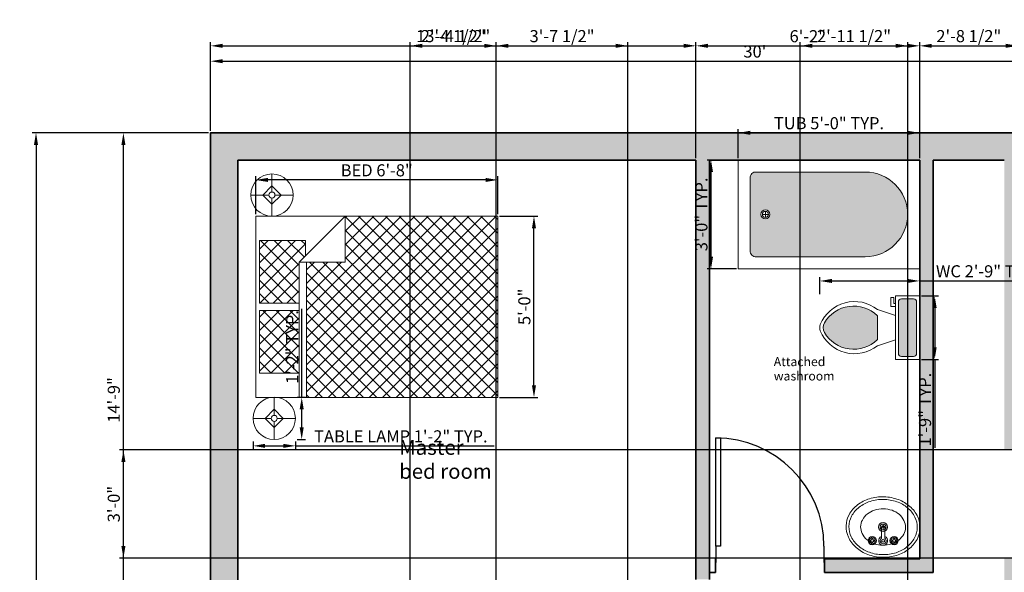
# Model space of a CAD drawing. Units: inches. Extents: x 1872 to 2380, y 714 to 1327.
# Tile 8 of 9: x 1872 to 2198, y 1144 to 1327. Entities that reach past the tile are written whole.
import ezdxf

# ---------------------------------------------------------------- set-up
doc = ezdxf.new("R2010")
doc.units = ezdxf.units.IN
for name, color, linetype, lineweight in [('A-ANNO-DIMS', 2, 'Continuous', 18), ('A-AREA-IDEN', 7, 'Continuous', 18), ('A-DOOR', 4, 'Continuous', 25), ('A-FLOR-FIXT', 9, 'Continuous', 20), ('A-FURN', 8, 'Continuous', 18), ('A-WALL', 7, 'Continuous', 35)]:
    doc.layers.add(name, color=color, linetype=linetype, lineweight=lineweight)
for name, color, linetype, lineweight, true_color in [('A-FLOR-FIXT-PATT', 7, 'Continuous', 13, 0xd1ffff), ('A-FURN-PATT', 254, 'Continuous', 13, 0xf8ceb3), ('A-WALL-PATT', 242, 'Continuous', 13, 0xd52e31)]:
    doc.layers.add(name, color=color, linetype=linetype, lineweight=lineweight, true_color=true_color)
doc.styles.get("Standard").update_dxf_attribs({"font": 'arial.ttf'})
doc.dimstyles.new('ISO-25', dxfattribs={"dimtxt": 4, "dimasz": 4, "dimexe": 1.25, "dimexo": 0.625, "dimtad": 1, "dimdec": 0, "dimlunit": 3, "dimtxsty": 'Standard', "dimcen": 2.5, "dimadec": 0, "dimazin": 0, "dimtfac": 1, "dimtdec": 0, "dimtmove": 0, "dimatfit": 3, "dimfxl": 1, "dimarcsym": 0})

# ---------------------------------------------------------------- blocks, each defined once
blk = doc.blocks.new('*U3')
for p, q in [((0, 0), (0, -6)), ((40, 0), (40, -6))]:
    blk.add_line(p, q)
blk.add_lwpolyline([(0, 0), (0, 40), (1.75, 40), (1.75, 0)], close=True)
blk.add_arc((0, 0), 40, 0, 90)
blk = doc.blocks.new('Bed - Queen')
for p, q in [((0, -80.00003), (0, 0)), ((0, 0), (59.99999, 0)), ((59.99999, 0), (59.99999, -80.00003)), ((7.99999, -1.2), (28.79998, -1.2)), ((7.99999, -14.4), (7.99999, -1.2)), ((28.79998, -1.2), (28.79998, -14.4)), ((31.19999, -1.2), (51.99999, -1.2)), ((31.19999, -14.4), (31.19999, -1.2)), ((51.99999, -1.2), (51.99999, -16.4)), ((0, -14.4), (44.8, -14.4)), ((59.99999, -29.6), (44.8, -14.4)), ((44.8, -14.4), (44.8, -29.6)), ((44.8, -16.8), (0, -16.8)), ((51.99999, -16.4), (46.79936, -16.4)), ((44.8, -29.6), (59.99999, -29.6)), ((59.99999, -80.00003), (0, -80.00003))]:
    blk.add_line(p, q)
blk = doc.blocks.new('Lamp - Table')
for p, q in [((0, 7), (0, 1)), ((-1, 0), (-7, 0)), ((0, 3), (-3, 0)), ((-3, 0), (0, -3)), ((3, 0), (0, 3)), ((0, -3), (3, 0)), ((1, 0), (7, 0)), ((0, -1), (0, -7))]:
    blk.add_line(p, q)
for radius in [7, 1]:
    blk.add_circle((0, 0), radius)
blk = doc.blocks.new('Bath Tub - 26 x 60 in.')
for p, q in [((8, -18), (10, -18)), ((9, -17), (9, -19))]:
    blk.add_line(p, q)
blk.add_lwpolyline([(0, -36), (0, 0), (60, 0), (60, -36)], close=True)
for points in [[(4, -30), (4, -6)], [(6, -4), (42, -4)], [(42, -32), (6, -32)]]:
    blk.add_lwpolyline(points)
for radius in [1.5, 1]:
    blk.add_circle((9, -18), radius)
for centre, radius, start, end in [((5.75, -5.75), 1.77, 81.8699, 188.1301), ((42, -18), 14, 270, 90), ((5.75, -30.25), 1.77, 171.8699, 278.1301)]:
    blk.add_arc(centre, radius, start, end)
blk = doc.blocks.new('Toilet - top')
for p, q in [((9.5, -6), (9.5, -2)), ((-10, -8.5), (-8, -8.5)), ((-10, -9.5), (-10, -8.5)), ((-7, -9.5), (-10, -9.5)), ((-8, -8.5), (-8, -8)), ((-7, -8), (-7, -9.5)), ((-4, -8), (-6, -14)), ((4, -8), (6, -14)), ((4, -14), (-4, -14))]:
    blk.add_line(p, q)
blk.add_lwpolyline([(10.5, -8), (10.5, 0), (-10.5, 0), (-10.5, -8)], close=True)
for points in [[(-9.5, -2), (-9.5, -6)], [(8.5, -1), (-8.5, -1)], [(-8.5, -7), (8.5, -7)]]:
    blk.add_lwpolyline(points)
for centre, radius, start, end in [((-8.62, -1.88), 0.884, 81.8699, 188.1301), ((8.62, -1.88), 0.884, 351.8699, 98.1301), ((-8.62, -6.12), 0.884, 171.8699, 278.1301), ((8.62, -6.12), 0.884, 261.8699, 8.1301), ((3.52, -21.58), 12.17, 141.4691, 247.9714), ((4.2, -21.82), 11.33, 136.3677, 238.9468), ((-3.52, -21.58), 12.17, 292.0284, 38.5307), ((-4.2, -21.82), 11.33, 301.053, 43.6321), ((0, -27.88), 4, 245.7318, 294.2682), ((0, -29), 4, 254.8605, 285.1395)]:
    blk.add_arc(centre, radius, start, end)
blk = doc.blocks.new('Sink - Oval top')
for p, q in [((-1, 0), (1, 0)), ((0, 1), (0, -1))]:
    blk.add_line(p, q)
for points in [[(-12.23, 0.39, 0.117634), (-11.46, -3.36, 0.104469), (-8.88, -6.8, 0.090016), (-5.08, -9.07, 0.08192), (-0.32, -10.02, 0.08192), (4.49, -9.38, 0.090016), (8.42, -7.36, 0.104469), (11.22, -4.09, 0.117634), (12.23, -0.39, 0.117634), (11.46, 3.36, 0.104469), (8.88, 6.8, 0.090016), (5.08, 9.07, 0.08192), (0.32, 10.02, 0.08192), (-4.49, 9.38, 0.090016), (-8.42, 7.36, 0.104469), (-11.22, 4.09, 0.117634)], [(-11.29, 0.16, 0.118622), (-10.52, -3.25, 0.104678), (-8.07, -6.36, 0.089562), (-4.54, -8.37, 0.081185), (-0.13, -9.15, 0.081185), (4.3, -8.49, 0.089562), (7.89, -6.58, 0.104678), (10.42, -3.55, 0.118622), (11.29, -0.16, 0.118622), (10.52, 3.25, 0.104678), (8.07, 6.36, 0.089562), (4.54, 8.37, 0.081185), (0.13, 9.15, 0.081185), (-4.3, 8.49, 0.089562), (-7.89, 6.58, 0.104678), (-10.42, 3.55, 0.118622)], [(-7.42, 0.08, 0.118283), (-6.91, -2.17, 0.104607), (-5.29, -4.21, 0.089718), (-2.97, -5.53, 0.081436), (-0.07, -6.04, 0.081436), (2.84, -5.59, 0.089718), (5.2, -4.33, 0.104607), (6.86, -2.32, 0.118283), (7.42, -0.08, 0.118283), (6.91, 2.17, 0.104607), (5.29, 4.21, 0.089718), (2.97, 5.53, 0.081436), (0.07, 6.04, 0.081436), (-2.84, 5.59, 0.089718), (-5.2, 4.33, 0.104607), (-6.86, 2.32, 0.118283)]]:
    blk.add_lwpolyline(points, format="xyb", close=True)
for radius in [1.5, 1]:
    blk.add_circle((0, 0), radius)
blk = doc.blocks.new('Faucet - Bathroom top')
for p, q in [((-4.107, 0.125), (-4.375, 0.125)), ((-3.75, 0.4788), (-3.75, 0.75)), ((-3.5, 0.482), (-3.5, 0.75)), ((-3.1461, 0.125), (-2.875, 0.125)), ((3.143, 0.125), (2.875, 0.125)), ((3.5, 0.4788), (3.5, 0.75)), ((3.75, 0.482), (3.75, 0.75)), ((4.1039, 0.125), (4.375, 0.125)), ((-4.1039, -0.125), (-4.375, -0.125)), ((-3.75, -0.4821), (-3.75, -0.75)), ((-3.5, -0.4789), (-3.5, -0.75)), ((-3.143, -0.125), (-2.875, -0.125)), ((-0.5, -0.8639), (-0.5, -4.5)), ((0.5, -4.5), (0.5, -0.8631)), ((3.1461, -0.125), (2.875, -0.125)), ((3.5, -0.4821), (3.5, -0.75)), ((3.75, -0.4789), (3.75, -0.75)), ((4.107, -0.125), (4.375, -0.125))]:
    blk.add_line(p, q)
for centre, radius in [((-3.625, 0), 1.375), ((-4.625, 0), 0.2795), ((-3.625, 0), 0.5), ((-3.625, 1), 0.2795), ((-2.625, 0), 0.2795), ((0, 0), 0.5), ((3.625, 0), 1.375), ((2.625, 0), 0.2795), ((3.625, 0), 0.5), ((3.625, 1), 0.2795), ((4.625, 0), 0.2795), ((-3.625, -1), 0.2795), ((3.625, -1), 0.2795)]:
    blk.add_circle(centre, radius)
for centre, radius, start, end in [((-3.625, 0), 1, 105.2407, 164.2093), ((-3.625, 0), 1, 16.44125, 74.07887), ((0, 0), 1.5, 289.6514, 250.3603), ((0, 0), 1, 300.3431, 239.7554), ((3.625, 0), 1, 106.12, 164.0884), ((3.625, 0), 1, 16.23422, 73.90469), ((-3.625, 0), 1, 196.2342, 253.9047), ((-3.625, 0), 1, 286.12, 344.0884), ((3.625, 0), 1, 196.4413, 254.0789), ((3.625, 0), 1, 285.2407, 344.2093), ((0, -4.5), 0.5, 180, 0)]:
    blk.add_arc(centre, radius, start, end)
blk = doc.blocks.new('*D22')
at = {"layer": 'A-ANNO-DIMS', "color": 0, "lineweight": -2, "transparency": 16777216}
for p, q in [((1935.4, 1290.27), (1935.4, 1314.61)), ((1939.4, 1313.36), (2291.4, 1313.36)), ((2295.4, 1290.27), (2295.4, 1314.61))]:
    blk.add_line(p, q, dxfattribs=at)
at = {"layer": 'A-ANNO-DIMS', "color": 0, "transparency": 16777216}
for points in [[(1939.4, 1314.03), (1939.4, 1312.69), (1935.4, 1313.36)], [(2291.4, 1314.03), (2291.4, 1312.69), (2295.4, 1313.36)]]:
    blk.add_solid(points, dxfattribs=at)
at = {"layer": 'Defpoints', "color": 0, "transparency": 16777216}
for p in [(2295.4, 1313.36), (1935.4, 1289.64), (2295.4, 1289.64)]:
    blk.add_point(p, dxfattribs=at)
at = {"layer": 'A-ANNO-DIMS', "color": 0, "transparency": 16777216, "insert": (2115.4, 1316.03), "char_height": 4, "attachment_point": 5}
blk.add_mtext("30'", dxfattribs=at)
blk = doc.blocks.new('*D23')
at = {"layer": 'A-ANNO-DIMS', "color": 0, "lineweight": -2, "transparency": 16777216}
for p, q in [((1934.77, 1289.64), (1876.44, 1289.64)), ((1877.69, 1285.64), (1877.69, 813.64)), ((1934.77, 809.64), (1876.44, 809.64))]:
    blk.add_line(p, q, dxfattribs=at)
at = {"layer": 'A-ANNO-DIMS', "color": 0, "transparency": 16777216}
for points in [[(1877.02, 1285.64), (1878.36, 1285.64), (1877.69, 1289.64)], [(1877.02, 813.64), (1878.36, 813.64), (1877.69, 809.64)]]:
    blk.add_solid(points, dxfattribs=at)
at = {"layer": 'Defpoints', "color": 0, "transparency": 16777216}
for p in [(1935.4, 1289.64), (1877.69, 809.64), (1935.4, 809.64)]:
    blk.add_point(p, dxfattribs=at)
at = {"layer": 'A-ANNO-DIMS', "color": 0, "transparency": 16777216, "insert": (1875.02, 1049.64), "char_height": 4, "attachment_point": 5, "rotation": 90}
blk.add_mtext("40'", dxfattribs=at)
blk = doc.blocks.new('*D24')
at = {"layer": 'A-ANNO-DIMS', "color": 0, "lineweight": -2, "transparency": 16777216}
for p, q in [((1949.46, 1187.48), (1949.46, 1184.76)), ((1953.46, 1186.01), (1959.46, 1186.01)), ((1963.46, 1187.48), (1963.46, 1184.76)), ((1963.46, 1186.01), (2029.21, 1186.01))]:
    blk.add_line(p, q, dxfattribs=at)
at = {"layer": 'A-ANNO-DIMS', "color": 0, "transparency": 16777216}
for points in [[(1953.46, 1186.68), (1953.46, 1185.34), (1949.46, 1186.01)], [(1959.46, 1186.68), (1959.46, 1185.34), (1963.46, 1186.01)]]:
    blk.add_solid(points, dxfattribs=at)
at = {"layer": 'Defpoints', "color": 0, "transparency": 16777216}
for p in [(1949.46, 1188.11), (1963.46, 1188.11), (1963.46, 1186.01)]:
    blk.add_point(p, dxfattribs=at)
at = {"layer": 'A-ANNO-DIMS', "color": 0, "transparency": 16777216, "insert": (1998.34, 1188.64), "char_height": 4, "attachment_point": 5}
blk.add_mtext('TABLE LAMP 1\'-2" TYP.', dxfattribs=at)
blk = doc.blocks.new('*D25')
at = {"layer": 'A-ANNO-DIMS', "color": 0, "lineweight": -2, "transparency": 16777216}
for p, q in [((1965.56, 1202.11), (1965.56, 1231.37)), ((1964.08, 1202.11), (1966.81, 1202.11)), ((1965.56, 1192.11), (1965.56, 1198.11)), ((1964.08, 1188.11), (1966.81, 1188.11))]:
    blk.add_line(p, q, dxfattribs=at)
at = {"layer": 'A-ANNO-DIMS', "color": 0, "transparency": 16777216}
for points in [[(1964.89, 1198.11), (1966.22, 1198.11), (1965.56, 1202.11)], [(1964.89, 1192.11), (1966.22, 1192.11), (1965.56, 1188.11)]]:
    blk.add_solid(points, dxfattribs=at)
at = {"layer": 'Defpoints', "color": 0, "transparency": 16777216}
for p in [(1963.46, 1202.11), (1965.56, 1202.11), (1963.46, 1188.11)]:
    blk.add_point(p, dxfattribs=at)
at = {"layer": 'A-ANNO-DIMS', "color": 0, "transparency": 16777216, "insert": (1962.92, 1218.74), "char_height": 4, "attachment_point": 5, "rotation": 90}
blk.add_mtext('1\'-2" TYP.', dxfattribs=at)
blk = doc.blocks.new('*D26')
at = {"layer": 'A-ANNO-DIMS', "color": 0, "lineweight": -2, "transparency": 16777216}
for p, q in [((1950.37, 1262.67), (1950.37, 1275.29)), ((2026.37, 1274.04), (1954.37, 1274.04)), ((2030.37, 1262.67), (2030.37, 1275.29))]:
    blk.add_line(p, q, dxfattribs=at)
at = {"layer": 'A-ANNO-DIMS', "color": 0, "transparency": 16777216}
for points in [[(1954.37, 1274.71), (1954.37, 1273.38), (1950.37, 1274.04)], [(2026.37, 1274.71), (2026.37, 1273.38), (2030.37, 1274.04)]]:
    blk.add_solid(points, dxfattribs=at)
at = {"layer": 'Defpoints', "color": 0, "transparency": 16777216}
for p in [(1950.37, 1274.04), (1950.37, 1262.04), (2030.37, 1262.04)]:
    blk.add_point(p, dxfattribs=at)
at = {"layer": 'A-ANNO-DIMS', "color": 0, "transparency": 16777216, "insert": (1990.37, 1276.71), "char_height": 4, "attachment_point": 5}
blk.add_mtext('BED 6\'-8"', dxfattribs=at)
blk = doc.blocks.new('*D27')
at = {"layer": 'A-ANNO-DIMS', "color": 0, "lineweight": -2, "transparency": 16777216}
for p, q in [((2030.99, 1262.04), (2043.62, 1262.04)), ((2042.37, 1206.04), (2042.37, 1258.04)), ((2030.99, 1202.04), (2043.62, 1202.04))]:
    blk.add_line(p, q, dxfattribs=at)
at = {"layer": 'A-ANNO-DIMS', "color": 0, "transparency": 16777216}
for points in [[(2041.7, 1258.04), (2043.03, 1258.04), (2042.37, 1262.04)], [(2041.7, 1206.04), (2043.03, 1206.04), (2042.37, 1202.04)]]:
    blk.add_solid(points, dxfattribs=at)
at = {"layer": 'Defpoints', "color": 0, "transparency": 16777216}
for p in [(2030.37, 1262.04), (2042.37, 1262.04), (2030.37, 1202.04)]:
    blk.add_point(p, dxfattribs=at)
at = {"layer": 'A-ANNO-DIMS', "color": 0, "transparency": 16777216, "insert": (2039.7, 1232.04), "char_height": 4, "attachment_point": 5, "rotation": 90}
blk.add_mtext('5\'-0"', dxfattribs=at)
blk = doc.blocks.new('*D34')
at = {"layer": 'A-ANNO-DIMS', "color": 0, "lineweight": -2, "transparency": 16777216}
for p, q in [((2109.91, 1281.27), (2109.91, 1290.89)), ((2113.91, 1289.64), (2165.91, 1289.64)), ((2169.91, 1281.27), (2169.91, 1290.89))]:
    blk.add_line(p, q, dxfattribs=at)
at = {"layer": 'A-ANNO-DIMS', "color": 0, "transparency": 16777216}
for points in [[(2113.91, 1290.31), (2113.91, 1288.98), (2109.91, 1289.64)], [(2165.91, 1290.31), (2165.91, 1288.98), (2169.91, 1289.64)]]:
    blk.add_solid(points, dxfattribs=at)
at = {"layer": 'Defpoints', "color": 0, "transparency": 16777216}
for p in [(2169.91, 1289.64), (2109.91, 1280.64), (2169.91, 1280.64)]:
    blk.add_point(p, dxfattribs=at)
at = {"layer": 'A-ANNO-DIMS', "color": 0, "transparency": 16777216, "insert": (2139.91, 1292.31), "char_height": 4, "attachment_point": 5}
blk.add_mtext('TUB 5\'-0" TYP.', dxfattribs=at)
blk = doc.blocks.new('*D35')
at = {"layer": 'A-ANNO-DIMS', "color": 0, "lineweight": -2, "transparency": 16777216}
for p, q in [((2109.29, 1280.64), (2099.66, 1280.64)), ((2100.91, 1248.64), (2100.91, 1276.64)), ((2109.29, 1244.64), (2099.66, 1244.64))]:
    blk.add_line(p, q, dxfattribs=at)
at = {"layer": 'A-ANNO-DIMS', "color": 0, "transparency": 16777216}
for points in [[(2100.25, 1276.64), (2101.58, 1276.64), (2100.91, 1280.64)], [(2100.25, 1248.64), (2101.58, 1248.64), (2100.91, 1244.64)]]:
    blk.add_solid(points, dxfattribs=at)
at = {"layer": 'Defpoints', "color": 0, "transparency": 16777216}
for p in [(2100.91, 1280.64), (2109.91, 1280.64), (2109.91, 1244.64)]:
    blk.add_point(p, dxfattribs=at)
at = {"layer": 'A-ANNO-DIMS', "color": 0, "transparency": 16777216, "insert": (2098.25, 1262.64), "char_height": 4, "attachment_point": 5, "rotation": 90}
blk.add_mtext('3\'-0" TYP.', dxfattribs=at)
blk = doc.blocks.new('*D36')
at = {"layer": 'A-ANNO-DIMS', "color": 0, "lineweight": -2, "transparency": 16777216}
for p, q in [((2136.87, 1236.27), (2136.87, 1241.85)), ((2140.87, 1240.6), (2165.91, 1240.6)), ((2169.91, 1236.27), (2169.91, 1241.85)), ((2169.91, 1240.6), (2210.57, 1240.6))]:
    blk.add_line(p, q, dxfattribs=at)
at = {"layer": 'A-ANNO-DIMS', "color": 0, "transparency": 16777216}
for points in [[(2140.87, 1241.27), (2140.87, 1239.93), (2136.87, 1240.6)], [(2165.91, 1241.27), (2165.91, 1239.93), (2169.91, 1240.6)]]:
    blk.add_solid(points, dxfattribs=at)
at = {"layer": 'Defpoints', "color": 0, "transparency": 16777216}
for p in [(2169.91, 1240.6), (2136.87, 1235.64), (2169.91, 1235.64)]:
    blk.add_point(p, dxfattribs=at)
at = {"layer": 'A-ANNO-DIMS', "color": 0, "transparency": 16777216, "insert": (2192.24, 1243.29), "char_height": 4, "attachment_point": 5}
blk.add_mtext('WC 2\'-9" TYP.', dxfattribs=at)
blk = doc.blocks.new('*D37')
at = {"layer": 'A-ANNO-DIMS', "color": 0, "lineweight": -2, "transparency": 16777216}
for p, q in [((2170.54, 1235.64), (2176.12, 1235.64)), ((2174.87, 1231.64), (2174.87, 1218.64)), ((2170.54, 1214.64), (2176.12, 1214.64)), ((2174.87, 1214.64), (2174.87, 1185.39))]:
    blk.add_line(p, q, dxfattribs=at)
at = {"layer": 'A-ANNO-DIMS', "color": 0, "transparency": 16777216}
for points in [[(2174.2, 1231.64), (2175.54, 1231.64), (2174.87, 1235.64)], [(2174.2, 1218.64), (2175.54, 1218.64), (2174.87, 1214.64)]]:
    blk.add_solid(points, dxfattribs=at)
at = {"layer": 'Defpoints', "color": 0, "transparency": 16777216}
for p in [(2169.91, 1235.64), (2169.91, 1214.64), (2174.87, 1214.64)]:
    blk.add_point(p, dxfattribs=at)
at = {"layer": 'A-ANNO-DIMS', "color": 0, "transparency": 16777216, "insert": (2172.2, 1198.01), "char_height": 4, "attachment_point": 5, "rotation": 90}
blk.add_mtext('1\'-9" TYP.', dxfattribs=at)
blk = doc.blocks.new('*D52')
at = {"layer": 'A-ANNO-DIMS', "color": 0, "lineweight": -2, "transparency": 16777216}
for p, q in [((1935.4, 1290.27), (1935.4, 1319.69)), ((2095.9, 1281.27), (2095.9, 1319.69)), ((1939.4, 1318.44), (2091.9, 1318.44))]:
    blk.add_line(p, q, dxfattribs=at)
at = {"layer": 'A-ANNO-DIMS', "color": 0, "transparency": 16777216}
for points in [[(1939.4, 1319.11), (1939.4, 1317.78), (1935.4, 1318.44)], [(2091.9, 1319.11), (2091.9, 1317.78), (2095.9, 1318.44)]]:
    blk.add_solid(points, dxfattribs=at)
at = {"layer": 'Defpoints', "color": 0, "transparency": 16777216}
for p in [(2095.9, 1318.44), (1935.4, 1289.64), (2095.9, 1280.64)]:
    blk.add_point(p, dxfattribs=at)
at = {"layer": 'A-ANNO-DIMS', "color": 0, "transparency": 16777216, "insert": (2015.65, 1321.14), "char_height": 4, "attachment_point": 5}
blk.add_mtext('13\'-4 1/2"', dxfattribs=at)
blk = doc.blocks.new('*D53')
at = {"layer": 'A-ANNO-DIMS', "color": 0, "lineweight": -2, "transparency": 16777216}
for p, q in [((2095.9, 1281.27), (2095.9, 1319.69)), ((2169.91, 1281.27), (2169.91, 1319.69)), ((2099.9, 1318.44), (2165.91, 1318.44))]:
    blk.add_line(p, q, dxfattribs=at)
at = {"layer": 'A-ANNO-DIMS', "color": 0, "transparency": 16777216}
for points in [[(2099.9, 1319.11), (2099.9, 1317.78), (2095.9, 1318.44)], [(2165.91, 1319.11), (2165.91, 1317.78), (2169.91, 1318.44)]]:
    blk.add_solid(points, dxfattribs=at)
at = {"layer": 'Defpoints', "color": 0, "transparency": 16777216}
for p in [(2169.91, 1318.44), (2095.9, 1280.64), (2169.91, 1280.64)]:
    blk.add_point(p, dxfattribs=at)
at = {"layer": 'A-ANNO-DIMS', "color": 0, "transparency": 16777216, "insert": (2132.91, 1321.11), "char_height": 4, "attachment_point": 5}
blk.add_mtext('6\'-2"', dxfattribs=at)
blk = doc.blocks.new('*D54')
at = {"layer": 'A-ANNO-DIMS', "color": 0, "lineweight": -2, "transparency": 16777216}
for p, q in [((2169.91, 1281.27), (2169.91, 1319.69)), ((2202.4, 1281.27), (2202.4, 1319.69)), ((2173.91, 1318.44), (2198.4, 1318.44))]:
    blk.add_line(p, q, dxfattribs=at)
at = {"layer": 'A-ANNO-DIMS', "color": 0, "transparency": 16777216}
for points in [[(2173.91, 1319.11), (2173.91, 1317.78), (2169.91, 1318.44)], [(2198.4, 1319.11), (2198.4, 1317.78), (2202.4, 1318.44)]]:
    blk.add_solid(points, dxfattribs=at)
at = {"layer": 'Defpoints', "color": 0, "transparency": 16777216}
for p in [(2202.4, 1318.44), (2169.91, 1280.64), (2202.4, 1280.64)]:
    blk.add_point(p, dxfattribs=at)
at = {"layer": 'A-ANNO-DIMS', "color": 0, "transparency": 16777216, "insert": (2186.16, 1321.14), "char_height": 4, "attachment_point": 5}
blk.add_mtext('2\'-8 1/2"', dxfattribs=at)
blk = doc.blocks.new('*D68')
at = {"layer": 'A-ANNO-DIMS', "color": 0, "lineweight": -2, "transparency": 16777216}
for p, q in [((1934.77, 1289.64), (1905.35, 1289.64)), ((1906.6, 1116.77), (1906.6, 1285.64)), ((1943.77, 1112.77), (1905.35, 1112.77))]:
    blk.add_line(p, q, dxfattribs=at)
at = {"layer": 'A-ANNO-DIMS', "color": 0, "transparency": 16777216}
for points in [[(1905.93, 1285.64), (1907.27, 1285.64), (1906.6, 1289.64)], [(1905.93, 1116.77), (1907.27, 1116.77), (1906.6, 1112.77)]]:
    blk.add_solid(points, dxfattribs=at)
at = {"layer": 'Defpoints', "color": 0, "transparency": 16777216}
for p in [(1906.6, 1289.64), (1935.4, 1289.64), (1944.4, 1112.77)]:
    blk.add_point(p, dxfattribs=at)
at = {"layer": 'A-ANNO-DIMS', "color": 0, "transparency": 16777216, "insert": (1903.93, 1201.21), "char_height": 4, "attachment_point": 5, "rotation": 90}
blk.add_mtext('14\'-9"', dxfattribs=at)
blk = doc.blocks.new('*D71')
at = {"layer": 'A-ANNO-DIMS', "color": 0, "lineweight": -2, "transparency": 16777216}
for p, q in [((2201.77, 1184.64), (1905.35, 1184.64)), ((1906.6, 1152.84), (1906.6, 1180.64)), ((2201.77, 1148.84), (1905.35, 1148.84))]:
    blk.add_line(p, q, dxfattribs=at)
at = {"layer": 'A-ANNO-DIMS', "color": 0, "transparency": 16777216}
for points in [[(1905.93, 1180.64), (1907.27, 1180.64), (1906.6, 1184.64)], [(1905.93, 1152.84), (1907.27, 1152.84), (1906.6, 1148.84)]]:
    blk.add_solid(points, dxfattribs=at)
at = {"layer": 'Defpoints', "color": 0, "transparency": 16777216}
for p in [(1906.6, 1184.64), (2202.4, 1184.64), (2202.4, 1148.84)]:
    blk.add_point(p, dxfattribs=at)
at = {"layer": 'A-ANNO-DIMS', "color": 0, "transparency": 16777216, "insert": (1903.93, 1166.74), "char_height": 4, "attachment_point": 5, "rotation": 90}
blk.add_mtext('3\'-0"', dxfattribs=at)
blk = doc.blocks.new('*D74')
at = {"layer": 'A-ANNO-DIMS', "color": 0, "lineweight": -2, "transparency": 16777216}
for p, q in [((2130.4, 953.62), (2130.4, 1319.69)), ((2166.01, 953.64), (2166.01, 1319.69)), ((2134.4, 1318.44), (2162.01, 1318.44))]:
    blk.add_line(p, q, dxfattribs=at)
at = {"layer": 'A-ANNO-DIMS', "color": 0, "transparency": 16777216}
for points in [[(2134.4, 1319.11), (2134.4, 1317.78), (2130.4, 1318.44)], [(2162.01, 1319.11), (2162.01, 1317.78), (2166.01, 1318.44)]]:
    blk.add_solid(points, dxfattribs=at)
at = {"layer": 'Defpoints', "color": 0, "transparency": 16777216}
for p in [(2166.01, 1318.44), (2130.4, 952.99), (2166.01, 953.01)]:
    blk.add_point(p, dxfattribs=at)
at = {"layer": 'A-ANNO-DIMS', "color": 0, "transparency": 16777216, "insert": (2148.2, 1321.14), "char_height": 4, "attachment_point": 5}
blk.add_mtext('2\'-11 1/2"', dxfattribs=at)
blk = doc.blocks.new('*D76')
at = {"layer": 'A-ANNO-DIMS', "color": 0, "lineweight": -2, "transparency": 16777216}
for p, q in [((2001.4, 953.62), (2001.4, 1319.69)), ((2029.9, 953.62), (2029.9, 1319.69)), ((2005.4, 1318.44), (2025.9, 1318.44))]:
    blk.add_line(p, q, dxfattribs=at)
at = {"layer": 'A-ANNO-DIMS', "color": 0, "transparency": 16777216}
for points in [[(2005.4, 1319.11), (2005.4, 1317.78), (2001.4, 1318.44)], [(2025.9, 1319.11), (2025.9, 1317.78), (2029.9, 1318.44)]]:
    blk.add_solid(points, dxfattribs=at)
at = {"layer": 'Defpoints', "color": 0, "transparency": 16777216}
for p in [(2029.9, 1318.44), (2001.4, 952.99), (2029.9, 952.99)]:
    blk.add_point(p, dxfattribs=at)
at = {"layer": 'A-ANNO-DIMS', "color": 0, "transparency": 16777216, "insert": (2015.65, 1321.14), "char_height": 4, "attachment_point": 5}
blk.add_mtext('2\'-4 1/2"', dxfattribs=at)
blk = doc.blocks.new('*D77')
at = {"layer": 'A-ANNO-DIMS', "color": 0, "lineweight": -2, "transparency": 16777216}
for p, q in [((2029.9, 953.62), (2029.9, 1319.69)), ((2073.4, 953.62), (2073.4, 1319.69)), ((2033.9, 1318.44), (2069.4, 1318.44))]:
    blk.add_line(p, q, dxfattribs=at)
at = {"layer": 'A-ANNO-DIMS', "color": 0, "transparency": 16777216}
for points in [[(2033.9, 1319.11), (2033.9, 1317.78), (2029.9, 1318.44)], [(2069.4, 1319.11), (2069.4, 1317.78), (2073.4, 1318.44)]]:
    blk.add_solid(points, dxfattribs=at)
at = {"layer": 'Defpoints', "color": 0, "transparency": 16777216}
for p in [(2073.4, 1318.44), (2029.9, 952.99), (2073.4, 952.99)]:
    blk.add_point(p, dxfattribs=at)
at = {"layer": 'A-ANNO-DIMS', "color": 0, "transparency": 16777216, "insert": (2051.65, 1321.14), "char_height": 4, "attachment_point": 5}
blk.add_mtext('3\'-7 1/2"', dxfattribs=at)

msp = doc.modelspace()

# ---------------------------------------------------------------- hatches: boundary and pattern name
at = {"layer": 'A-FLOR-FIXT-PATT', "transparency": 33554687}
h = msp.add_hatch(color=256, dxfattribs=at)
h.dxf.hatch_style = 1
h.paths.add_polyline_path([(2244.4, 1008.14), (2208.4, 1008.14, 0.5), (2206.4, 1006.14), (2206.4, 982.14, 0.5), (2208.4, 980.14), (2244.4, 980.14, 1)])
h.paths.add_polyline_path([(2209.9, 994.14, -1), (2212.9, 994.14, -1)], flags=16)
h.paths.add_polyline_path([(2210.4, 994.14, -1), (2212.4, 994.14, -1)], flags=0)
h.paths.add_polyline_path([(2151.91, 1276.64), (2115.91, 1276.64, 0.5), (2113.91, 1274.64), (2113.91, 1250.64, 0.5), (2115.91, 1248.64), (2151.91, 1248.64, 1)])
h.paths.add_polyline_path([(2117.41, 1262.64, -1), (2120.41, 1262.64, -1)], flags=16)
h.paths.add_polyline_path([(2117.91, 1262.64, -1), (2119.91, 1262.64, -1)], flags=0)
h = msp.add_hatch(color=256, dxfattribs=at)
h.dxf.hatch_style = 1
h.paths.add_polyline_path([(2155.91, 1229.14, 0.48008), (2138.39, 1226.79, 0.215004), (2138.39, 1223.5, 0.48008), (2155.91, 1221.14)])
h.paths.add_polyline_path([(2168.91, 1233.64, 0.5), (2167.91, 1234.64), (2163.91, 1234.64, 0.5), (2162.91, 1233.64), (2162.91, 1216.64, 0.5), (2163.91, 1215.64), (2167.91, 1215.64, 0.5), (2168.91, 1216.64)])
h.paths.add_polyline_path([(2285.4, 982.14, 0.5), (2284.4, 983.14), (2267.4, 983.14, 0.5), (2266.4, 982.14), (2266.4, 978.14, 0.5), (2267.4, 977.14), (2284.4, 977.14, 0.5), (2285.4, 978.14)])
h.paths.add_polyline_path([(2277.54, 1007.66, 0.215004), (2274.25, 1007.66, 0.48008), (2271.9, 990.14), (2279.9, 990.14, 0.48008)])
h.paths.add_polyline_path([(2285.9, 985.64), (2282.9, 985.64), (2282.9, 984.14), (2283.9, 984.14), (2283.9, 984.64), (2285.9, 984.64)])
h.paths.add_polyline_path([(2279.53, 1049.02, -0.039819), (2280.2, 1048.28, 0.216904), (2280.37, 1048.66, 0.658258)])
h.paths.add_polyline_path([(2279.53, 1049.02, 0.206085), (2279.37, 1048.66, 0.643515), (2280.2, 1048.28, 0.039819)])
h.paths.add_polyline_path([(2279.37, 1045.03, 1), (2280.37, 1045.03, 1)])
h.paths.add_polyline_path([(2280.37, 1041.41, 0.219955), (2280.19, 1041.79, -0.039801), (2279.52, 1041.05, 0.66578)])
h.paths.add_polyline_path([(2280.19, 1041.79, 0.639405), (2279.37, 1041.41, 0.200639), (2279.52, 1041.05, 0.039801)])
h.paths.add_polyline_path([(2158.34, 1154.61, 1), (2157.34, 1154.61, 1)])
h.paths.add_polyline_path([(2154.72, 1154.61, 1), (2153.72, 1154.61, 1)])
h.paths.add_polyline_path([(2161.97, 1154.61, 1), (2160.97, 1154.61, 1)])
h.paths.add_polyline_path([(2180.69, 824, 1), (2181.69, 824, 1)])
h.paths.add_polyline_path([(2185.32, 824, 1), (2184.32, 824, 1)])
h.paths.add_polyline_path([(2188.94, 824, 1), (2187.94, 824, 1)])
at = {"layer": 'A-FURN-PATT', "transparency": 33554687}
h = msp.add_hatch(dxfattribs=at)
h.set_pattern_fill('ANSI37', color=256)
h.paths.add_polyline_path([(2030.37, 1262.04), (1979.97, 1262.04), (1979.97, 1246.84), (1967.17, 1246.84), (1967.17, 1202.04), (2030.37, 1202.04)])
h.paths.add_polyline_path([(1964.77, 1246.84), (1966.77, 1248.84), (1966.77, 1254.04), (1951.57, 1254.04), (1951.57, 1233.24), (1964.77, 1233.24)])
h.paths.add_polyline_path([(1964.77, 1230.84), (1951.57, 1230.84), (1951.57, 1210.04), (1964.77, 1210.04)])
h.paths.add_polyline_path([(2268.08, 1263.68), (2221.12, 1263.68), (2221.12, 1219.09), (2258.57, 1219.09), (2258.57, 1230.39), (2268.08, 1230.39)])
h.paths.add_polyline_path([(2279.67, 1257.73), (2269.86, 1257.73), (2269.86, 1242.28), (2279.67, 1242.28)])
h.paths.add_polyline_path([(2279.67, 1240.49), (2269.86, 1240.49), (2269.86, 1230.39), (2268.38, 1228.9), (2268.38, 1225.04), (2279.67, 1225.04)])
h.paths.add_polyline_path([(2097.97, 1011.83), (2085.54, 1011.83), (2085.42, 1011.06), (2098.09, 1011.06)])
h.paths.add_polyline_path([(2098.15, 1010.67), (2085.36, 1010.67), (2084.39, 1004.45), (2099.13, 1004.45)])
h.paths.add_polyline_path([(2119.91, 1010.67), (2107.12, 1010.67), (2106.14, 1004.45), (2120.89, 1004.45)])
h.paths.add_polyline_path([(2119.73, 1011.83), (2107.3, 1011.83), (2107.18, 1011.06), (2119.85, 1011.06)])
h.paths.add_polyline_path([(2074.66, 997.83), (2068.44, 996.86), (2068.44, 984.06), (2074.66, 983.09)])
h.paths.add_polyline_path([(2068.05, 996.8), (2067.28, 996.68), (2067.28, 984.25), (2068.05, 984.12)])
h.paths.add_polyline_path([(2136.83, 996.86), (2130.61, 997.83), (2130.61, 983.09), (2136.83, 984.06)])
h.paths.add_polyline_path([(2137.99, 996.68), (2137.22, 996.8), (2137.22, 984.12), (2137.99, 984.25)])
h.paths.add_polyline_path([(2099.13, 976.47), (2084.39, 976.47), (2085.36, 970.26), (2098.15, 970.26)])
h.paths.add_polyline_path([(2120.89, 976.47), (2106.14, 976.47), (2107.12, 970.26), (2119.91, 970.26)])
h.paths.add_polyline_path([(2119.85, 969.87), (2107.18, 969.87), (2107.3, 969.09), (2119.73, 969.09)])
h.paths.add_polyline_path([(2098.09, 969.87), (2085.42, 969.87), (2085.54, 969.09), (2097.97, 969.09)])
at = {"layer": 'A-WALL-PATT', "transparency": 33554687}
h = msp.add_hatch(color=256, dxfattribs=at)
h.dxf.hatch_style = 1
h.paths.add_polyline_path([(2295.4, 1289.64), (1935.4, 1289.64), (1935.4, 809.64), (1949.4, 809.64), (1949.4, 818.64), (1944.4, 818.64), (1944.4, 1108.27), (2100.4, 1108.27), (2100.4, 1112.77), (1944.4, 1112.77), (1944.4, 1280.64), (2095.9, 1280.64), (2095.9, 1141.77), (2100.4, 1141.77), (2100.4, 1280.64), (2169.91, 1280.64), (2169.91, 1244.64), (2169.91, 1160.49, -0.053008), (2170.04, 1158.75, -0.03687), (2169.91, 1157.54), (2169.91, 1148.64), (2167.91, 1148.64), (2138.4, 1148.64), (2138.4, 1144.14), (2167.91, 1144.14), (2174.41, 1144.14), (2174.41, 1280.64), (2197.9, 1280.64), (2197.9, 1184.64), (2202.4, 1184.64), (2202.4, 1280.64), (2286.4, 1280.64), (2286.4, 1148.64), (2197.9, 1148.64), (2197.9, 1108.14), (2202.4, 1108.14), (2202.4, 1144.14), (2286.4, 1144.14), (2286.4, 1060.14), (2202.4, 1060.14), (2202.4, 1108.14), (2197.9, 1108.14), (2197.9, 1060.14), (2197.9, 1053.64), (2202.4, 1053.64), (2202.4, 1055.64), (2286.4, 1055.64), (2286.4, 976.14), (2202.4, 976.14), (2202.4, 1015.64), (2197.9, 1015.64), (2197.9, 971.64), (2197.9, 952.99), (2197.9, 818.64), (2101.9, 818.64), (2101.9, 948.71), (2130.4, 948.71), (2130.4, 952.99), (2073.4, 952.99), (2073.4, 948.71), (2097.4, 948.71), (2097.4, 818.64), (2005.9, 818.64), (2005.9, 948.71), (2029.9, 948.71), (2029.9, 952.99), (2001.4, 952.99), (2001.4, 818.64), (1996.4, 818.64), (1985.23, 818.64), (1985.23, 809.64), (1996.4, 809.64), (2295.4, 809.64)])
h.paths.add_polyline_path([(2202.4, 971.64), (2286.4, 971.64), (2286.4, 858.19), (2286.62, 858.19), (2286.62, 857.19), (2286.4, 857.19), (2286.4, 828.68), (2286.48, 828.76), (2286.4, 828.43), (2286.4, 818.64), (2256.29, 818.64), (2255.29, 818.39), (2254.54, 818.64), (2238.99, 818.64), (2238.75, 818.58), (2238.56, 818.64), (2202.4, 818.64), (2202.4, 952.99)], flags=16)
h.paths.add_polyline_path([(2260.41, 970, -0.15), (2280.41, 970), (2278.41, 967, 0.001913), (2277.92, 967.06), (2277.41, 964.5), (2278.64, 964.5), (2278.72, 964), (2279.41, 964), (2282.41, 953, -0.541163), (2280.76, 950.93), (2280.91, 950, -0.414214), (2279.91, 949), (2279.41, 949), (2279.91, 945), (2278.41, 945), (2277.91, 949), (2270.41, 949), (2262.91, 949), (2262.41, 945), (2260.91, 945), (2261.41, 949), (2260.91, 949, -0.414214), (2259.91, 950), (2260.05, 950.93, -0.505809), (2258.36, 952.83), (2261.41, 964), (2262.1, 964), (2262.17, 964.5), (2263.41, 964.5), (2262.9, 967.06, 0.001913), (2262.41, 967)], flags=0)
h.paths.add_polyline_path([(2257.85, 934.42), (2280.51, 934.42, -0.333333), (2281.77, 933.16), (2281.77, 923.09, -0.333333), (2280.51, 921.83), (2277.57, 921.83), (2277.57, 921.41), (2275.89, 921.41), (2275.89, 921.83), (2262.46, 921.83), (2262.46, 921.41), (2260.79, 921.41), (2260.79, 921.83), (2257.85, 921.83, -0.333333), (2256.59, 923.09), (2256.59, 933.16, -0.333333)], flags=0)
h.paths.add_polyline_path([(2260.61, 912.79), (2262.11, 912.79), (2262.61, 908.79), (2270.11, 908.79), (2277.61, 908.79), (2278.11, 912.79), (2279.61, 912.79), (2279.11, 908.79), (2279.61, 908.79, -0.414214), (2280.61, 907.79), (2280.46, 906.86, -0.505809), (2282.15, 904.96), (2279.11, 893.79), (2278.42, 893.79), (2278.34, 893.29), (2277.11, 893.29), (2277.62, 890.73, 0.001913), (2278.11, 890.79), (2280.11, 887.79, -0.15), (2260.11, 887.79), (2262.11, 890.79, 0.001913), (2262.59, 890.73), (2263.11, 893.29), (2261.87, 893.29), (2261.79, 893.79), (2261.11, 893.79), (2258.11, 904.79, -0.541163), (2259.75, 906.86), (2259.61, 907.79, -0.414214), (2260.61, 908.79), (2261.11, 908.79)], flags=0)
h.paths.add_polyline_path([(2252.62, 864.69), (2253.62, 864.69), (2253.62, 862.19), (2253.62, 860.69), (2256.62, 859.69, -0.362186), (2259.62, 862.19, -0.174416), (2262.62, 860.69, 0.103487), (2265.62, 859.19, -0.219276), (2266.55, 858.19), (2268.62, 858.19), (2268.62, 859.69), (2267.62, 859.69), (2267.62, 863.69), (2270.12, 863.69), (2270.12, 859.69), (2269.12, 859.69), (2269.12, 858.19), (2274.62, 858.19), (2278.62, 858.19), (2278.62, 862.69), (2275.62, 864.69), (2275.62, 865.69), (2279.62, 862.69), (2279.62, 858.19), (2279.62, 852.69), (2275.62, 849.19), (2275.62, 850.19), (2278.62, 852.69), (2278.62, 857.19), (2274.62, 857.19), (2271.12, 857.19), (2271.12, 855.69), (2272.12, 855.69), (2272.12, 851.69), (2269.62, 851.69), (2269.62, 855.69), (2270.62, 855.69), (2270.62, 857.19), (2266.55, 857.19, -0.219162), (2265.62, 856.19, 0.103506), (2262.62, 854.69, -0.174459), (2259.62, 853.19, -0.362114), (2256.62, 855.69), (2253.62, 854.69), (2253.62, 850.69), (2252.62, 850.69)], flags=0)
h.paths.add_polyline_path([(2253.62, 859.69), (2256.62, 858.69), (2256.62, 856.69), (2253.62, 855.69)], flags=0)
h.paths.add_polyline_path([(2208.62, 838.17), (2208.28, 836.61), (2207.75, 836.18), (2207.67, 833.93), (2208.71, 832.96), (2211.55, 836.09), (2214.43, 837.53), (2214.45, 837.55), (2214.61, 836.16), (2215.48, 834.9), (2215.87, 835.13), (2217.12, 836.79), (2216.83, 834.17), (2218.8, 828.76), (2219.23, 829.13), (2220.06, 831.53), (2219.5, 837.61), (2219.53, 837.66), (2219.68, 838.72), (2219.62, 838.91), (2219.72, 839.01), (2219.51, 837.47), (2219.77, 834.68), (2220.87, 834.05), (2221.03, 834.58), (2222.05, 835.47), (2222.71, 834.65), (2223.67, 836.89), (2224.63, 836.57), (2226.23, 835.08), (2227.55, 836.18), (2227.59, 837.16), (2228.42, 838.17), (2228.08, 836.61), (2227.55, 836.18), (2227.47, 833.93), (2228.51, 832.96), (2231.35, 836.09), (2234.23, 837.53), (2234.25, 837.55), (2234.42, 836.16), (2235.28, 834.9), (2235.67, 835.13), (2236.93, 836.79), (2236.93, 836.84), (2238.69, 834.65), (2239.41, 836.34), (2239.3, 837.61), (2239.34, 837.66), (2239.48, 838.72), (2239.42, 838.91), (2239.52, 839.01), (2239.31, 837.47), (2239.36, 836.98), (2240.61, 836.57), (2242.2, 835.08), (2243.53, 836.18), (2243.57, 837.16), (2244.39, 838.17), (2244.05, 836.61), (2243.53, 836.18), (2243.44, 833.93), (2244.49, 832.96), (2247.33, 836.09), (2250.21, 837.53), (2250.22, 837.55), (2250.39, 836.16), (2251.25, 834.9), (2251.65, 835.13), (2252.9, 836.79), (2252.61, 834.17), (2254.09, 830.08), (2254.54, 829.37), (2254.85, 828.99), (2255.01, 829.13), (2255.83, 831.53), (2255.29, 837.44), (2255.28, 837.44), (2255.46, 838.72), (2255.4, 838.91), (2255.5, 839.01), (2255.28, 837.47), (2255.29, 837.44), (2257.9, 836.57), (2259.5, 835.08), (2260.82, 836.18), (2260.86, 837.16), (2261.69, 838.17), (2261.35, 836.61), (2260.82, 836.18), (2260.74, 833.93), (2261.78, 832.96), (2264.62, 836.09), (2267.5, 837.53), (2267.52, 837.55), (2267.68, 836.16), (2268.54, 834.9), (2268.94, 835.13), (2270.19, 836.79), (2269.9, 834.17), (2271.79, 828.96), (2271.98, 828.86), (2272.3, 829.13), (2273.13, 831.53), (2272.56, 837.61), (2272.6, 837.66), (2272.75, 838.72), (2272.69, 838.91), (2272.79, 839.01), (2272.58, 837.47), (2273.13, 831.53), (2273.02, 831.22), (2273.67, 831.01), (2273.92, 831.6), (2273.83, 830.95), (2274.1, 830.86), (2275.75, 833.35), (2276.03, 831.86), (2276.57, 831.38), (2277, 831.91), (2277.3, 833.27), (2279.06, 830.44), (2281.09, 831.46), (2281.1, 831.48), (2281.21, 830.5), (2281.82, 829.61), (2282.1, 829.77), (2282.98, 830.94), (2282.77, 829.1), (2284.15, 825.3), (2284.46, 825.55), (2285.04, 827.24), (2284.64, 831.51), (2284.67, 831.55), (2284.77, 832.3), (2284.73, 832.43), (2284.8, 832.5), (2284.65, 831.42), (2285.04, 827.24), (2284.46, 825.55), (2283.45, 824.71), (2281.76, 819.99), (2278.73, 818.64), (2276.7, 819.65), (2275.69, 821.34), (2274.34, 822.01), (2272.32, 824.04), (2269.58, 824.33), (2268.46, 821.21), (2264.14, 819.29), (2261.26, 820.73), (2259.82, 823.13), (2257.9, 824.09), (2255.02, 826.97), (2253.29, 827.15), (2251.17, 821.21), (2246.85, 819.29), (2243.97, 820.73), (2242.53, 823.13), (2240.61, 824.09), (2237.73, 826.97), (2237.27, 827.01), (2235.19, 821.21), (2230.87, 819.29), (2227.99, 820.73), (2226.55, 823.13), (2224.63, 824.09), (2221.75, 826.97), (2217.61, 827.41), (2215.39, 821.21), (2211.07, 819.29), (2208.19, 820.73), (2206.75, 823.13), (2204.83, 824.09), (2203.87, 826.49), (2202.91, 830.81), (2202.91, 834.65), (2203.87, 836.89), (2204.83, 836.57), (2206.43, 835.08), (2207.75, 836.18), (2207.79, 837.16)], flags=0)
h.paths.add_polyline_path([(2221.04, 832.88), (2221.82, 832.52), (2222.11, 833.69), (2222.71, 834.29), (2222.71, 832.11), (2225.59, 830.81), (2226.55, 830.81), (2228.95, 822.65), (2230.87, 820.25), (2230.87, 819.29), (2233.27, 821.21), (2233.75, 823.61), (2232.79, 826.97), (2231.99, 830.19), (2236.41, 827.71), (2236.63, 831.29), (2235.93, 834.58), (2242.53, 830.81), (2241.57, 830.81), (2240.97, 831.07), (2240.47, 830.33), (2239.06, 829.14), (2239.65, 826.49), (2237.25, 829.37), (2236.52, 829.55), (2236.41, 827.71), (2231.99, 830.19), (2232.79, 826.97), (2233.75, 823.61), (2233.27, 821.21), (2230.87, 819.29), (2230.87, 820.25), (2228.95, 822.65), (2226.55, 830.81), (2225.59, 830.81), (2222.71, 832.11), (2222.71, 830.81), (2223.67, 826.49), (2221.27, 829.37), (2220.67, 830.33), (2220.67, 830.33)], flags=0)
h.paths.add_polyline_path([(2255.98, 833), (2259.82, 830.81), (2258.86, 830.81), (2257.25, 831.54), (2256.45, 830.33), (2256.66, 831.81), (2256.02, 832.1), (2255.98, 831.99)], flags=0)
h.paths.add_polyline_path([(2275.69, 826.73), (2277.07, 828.25), (2275.46, 829.74), (2276.39, 830.51), (2276.33, 828.93), (2279.06, 826.4), (2278.73, 823.36), (2277.38, 821)], flags=0)
h.paths.add_polyline_path([(2260.6, 925.25), (2276.34, 925.25), (2276.34, 931.01), (2260.6, 931.01)], flags=8)
h.paths.add_polyline_path([(2202.72, 1070.05), (2202.72, 1092.72), (2197.34, 1092.72), (2197.34, 1070.05)], flags=25)

# ---------------------------------------------------------------- linework, layer by layer
at = {"layer": 'A-WALL'}
for p, q in [((1944.4, 1280.64), (2095.9, 1280.64)), ((2095.9, 1141.77), (2095.9, 1280.64)), ((2100.4, 1141.77), (2100.4, 1280.64)), ((2169.91, 1280.64), (2169.91, 1148.64)), ((2174.41, 1280.64), (2174.41, 1144.14)), ((2102.4, 1144.14), (2102.4, 1148.64)), ((2138.4, 1144.14), (2138.4, 1148.64)), ((2138.4, 1148.64), (2167.91, 1148.64)), ((2167.91, 1148.64), (2169.91, 1148.64)), ((2100.4, 1144.14), (2102.4, 1144.14)), ((2138.4, 1144.14), (2167.91, 1144.14)), ((2167.91, 1144.14), (2174.41, 1144.14))]:
    msp.add_line(p, q, dxfattribs=at)
at = {"layer": 'A-WALL', "transparency": 33554687}
for p, q in [((1944.4, 1112.77), (1944.4, 1280.64)), ((2100.4, 1280.64), (2169.91, 1280.64)), ((2174.41, 1280.64), (2197.9, 1280.64))]:
    msp.add_line(p, q, dxfattribs=at)
msp.add_lwpolyline([(1949.4, 809.64), (1935.4, 809.64), (1935.4, 1289.64), (2295.4, 1289.64), (2295.4, 809.64), (1996.4, 809.64)], dxfattribs=at)

# ---------------------------------------------------------------- block references
at = {"layer": 'A-DOOR', "xscale": 0.895133583936691, "yscale": 0.895133583936691, "zscale": 0.895133583936691}
msp.add_blockref('*U3', (2102.46, 1152.81), dxfattribs=at)
at = {"layer": 'A-FLOR-FIXT', "transparency": 33554687}
for name, p in [('Bath Tub - 26 x 60 in.', (2109.91, 1280.64)), ('Sink - Oval top', (2157.81, 1159.14))]:
    msp.add_blockref(name, p, dxfattribs=at)
for name, p, rotation in [('Toilet - top', (2169.91, 1225.14), 270), ('Faucet - Bathroom top', (2157.84, 1154.61), 180)]:
    msp.add_blockref(name, p, dxfattribs=dict(at, rotation=rotation))
at = {"layer": 'A-FURN', "transparency": 33554687}
for p in [(1955.72, 1269.04), (1956.46, 1195.11)]:
    msp.add_blockref('Lamp - Table', p, dxfattribs=at)
at = {"layer": 'A-FURN', "transparency": 33554687, "rotation": 90}
msp.add_blockref('Bed - Queen', (1950.37, 1202.04), dxfattribs=at)

# ---------------------------------------------------------------- texts
at = {"layer": 'A-AREA-IDEN', "transparency": 33554687}
for s, height, p in [('Attached ', 2.965, (2121.66, 1212.41)), ('washroom ', 2.965, (2121.66, 1207.65)), ('Master ', 4.939, (1997.79, 1183.05)), ('bed room', 4.939, (1997.79, 1175.11))]:
    msp.add_text(s, height=height, dxfattribs=at).set_placement(p)

# ---------------------------------------------------------------- dimensions: what is measured, and where the dimension line sits
at = {"layer": 'A-ANNO-DIMS', "transparency": 33554687}
for base, p1, p2, override, picture, middle in [((2095.9, 1318.44), (1935.4, 1289.64), (2095.9, 1280.64), {"dimdec": 1, "dimlfac": 1, "dimrnd": 0, "dimzin": 1, "dimdsep": 46, "dimlunit": 4, "dimfrac": 2}, '*D52', (2015.65, 1321.14)), ((2029.9, 1318.44), (2001.4, 952.99), (2029.9, 952.99), {"dimdec": 1, "dimlfac": 1, "dimrnd": 0, "dimzin": 1, "dimdsep": 46, "dimlunit": 4, "dimfrac": 2}, '*D76', (2015.65, 1321.14)), ((2073.4, 1318.44), (2029.9, 952.99), (2073.4, 952.99), {"dimdec": 1, "dimlfac": 1, "dimrnd": 0, "dimzin": 1, "dimdsep": 46, "dimlunit": 4, "dimfrac": 2}, '*D77', (2051.65, 1321.14)), ((2166.01, 1318.44), (2130.4, 952.99), (2166.01, 953.01), {"dimdec": 1, "dimlfac": 1, "dimrnd": 0, "dimzin": 1, "dimdsep": 46, "dimlunit": 4, "dimfrac": 2}, '*D74', (2148.2, 1321.14)), ((2202.4, 1318.44), (2169.91, 1280.64), (2202.4, 1280.64), {"dimdec": 1, "dimlfac": 1, "dimrnd": 0, "dimzin": 1, "dimdsep": 46, "dimlunit": 4, "dimfrac": 2}, '*D54', (2186.16, 1321.14)), ((2169.91, 1318.44), (2095.9, 1280.64), (2169.91, 1280.64), {"dimdec": 1, "dimlfac": 1, "dimrnd": 0, "dimzin": 1, "dimdsep": 46, "dimlunit": 4, "dimfrac": 2}, '*D53', (2132.91, 1321.11)), ((2295.4, 1313.36), (1935.4, 1289.64), (2295.4, 1289.64), {"dimclrd": 0, "dimclre": 0, "dimclrt": 0}, '*D22', (2115.4, 1316.03))]:
    dim = msp.add_linear_dim(base=base, p1=p1, p2=p2, dimstyle='ISO-25', override=override, dxfattribs=at)
    dim.commit()
    dim.dimension.update_dxf_attribs({"geometry": picture, "text_midpoint": middle})
for base, p1, p2, text, picture, middle in [((2169.91, 1289.64), (2109.91, 1280.64), (2169.91, 1280.64), 'TUB <> TYP.', '*D34', (2139.91, 1292.31)), ((2169.91, 1240.6), (2136.87, 1235.64), (2169.91, 1235.64), 'WC <> TYP.', '*D36', (2192.24, 1243.29)), ((1963.46, 1186.01), (1949.46, 1188.11), (1963.46, 1188.11), 'TABLE LAMP <> TYP.', '*D24', (1998.34, 1188.64))]:
    dim = msp.add_linear_dim(base=base, p1=p1, p2=p2, text=text, dimstyle='ISO-25', override={"dimdec": 1, "dimlfac": 1, "dimrnd": 0, "dimzin": 1, "dimdsep": 46, "dimlunit": 4, "dimfrac": 2}, dxfattribs=at)
    dim.commit()
    dim.dimension.update_dxf_attribs({"geometry": picture, "text_midpoint": middle})
for base, p1, p2, override, picture, middle in [((1877.69, 809.64), (1935.4, 1289.64), (1935.4, 809.64), {"dimclrd": 0, "dimclre": 0, "dimclrt": 0}, '*D23', (1875.02, 1049.64)), ((1906.6, 1289.64), (1944.4, 1112.77), (1935.4, 1289.64), {"dimdec": 1, "dimlfac": 1, "dimrnd": 0, "dimzin": 1, "dimdsep": 46, "dimlunit": 4, "dimfrac": 2}, '*D68', (1903.93, 1201.21)), ((2042.37, 1262.04), (2030.37, 1202.04), (2030.37, 1262.04), {"dimdec": 1, "dimlfac": 1, "dimrnd": 0, "dimzin": 1, "dimdsep": 46, "dimlunit": 4, "dimfrac": 2}, '*D27', (2039.7, 1232.04)), ((1906.6, 1184.64), (2202.4, 1148.84), (2202.4, 1184.64), {"dimdec": 1, "dimlfac": 1, "dimrnd": 0, "dimzin": 1, "dimdsep": 46, "dimlunit": 4, "dimfrac": 2}, '*D71', (1903.93, 1166.74))]:
    dim = msp.add_linear_dim(base=base, p1=p1, p2=p2, angle=90, dimstyle='ISO-25', override=override, dxfattribs=at)
    dim.commit()
    dim.dimension.update_dxf_attribs({"geometry": picture, "text_midpoint": middle})
for base, p1, p2, angle, text, picture, middle in [((1950.37, 1274.04), (2030.37, 1262.04), (1950.37, 1262.04), 180, 'BED <>', '*D26', (1990.37, 1276.71)), ((2100.91, 1280.64), (2109.91, 1244.64), (2109.91, 1280.64), 90, '<> TYP.', '*D35', (2098.25, 1262.64)), ((2174.87, 1214.64), (2169.91, 1235.64), (2169.91, 1214.64), 270, '<> TYP.', '*D37', (2172.2, 1198.01)), ((1965.56, 1202.11), (1963.46, 1188.11), (1963.46, 1202.11), 90, '<> TYP.', '*D25', (1962.92, 1218.74))]:
    dim = msp.add_linear_dim(base=base, p1=p1, p2=p2, angle=angle, text=text, dimstyle='ISO-25', override={"dimdec": 1, "dimlfac": 1, "dimrnd": 0, "dimzin": 1, "dimdsep": 46, "dimlunit": 4, "dimfrac": 2}, dxfattribs=at)
    dim.commit()
    dim.dimension.update_dxf_attribs({"geometry": picture, "text_midpoint": middle})

doc.saveas('drawing.dxf')
